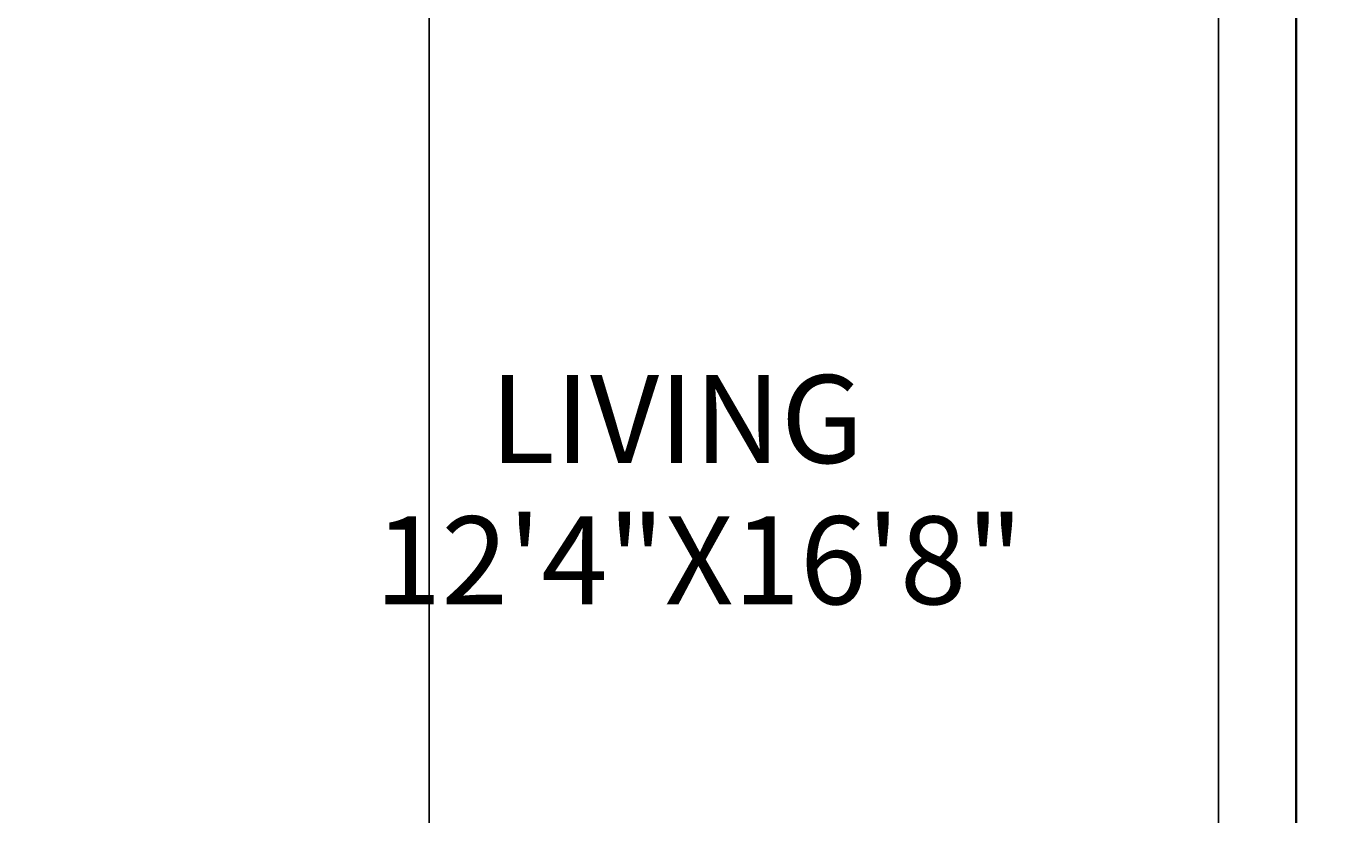
# Model space of a CAD drawing. Units: feet. Extents: x 5816 to 6644, y 25475 to 26788.
# Tile 9 of 23: x 6052 to 6232, y 26265 to 26373. Entities that reach past the tile are written whole.
import ezdxf

# ---------------------------------------------------------------- set-up
doc = ezdxf.new("R2010")
doc.units = ezdxf.units.FT
for name, color, linetype, lineweight in [('A-ANNO-DIMS', 2, 'Continuous', 13), ('A-AREA-IDEN', 7, 'Continuous', 18), ('A-WALL', 7, 'Continuous', 35)]:
    doc.layers.add(name, color=color, linetype=linetype, lineweight=lineweight)
doc.styles.get("Standard").update_dxf_attribs({"font": 'arial.ttf'})
doc.dimstyles.get("Standard").update_dxf_attribs({"dimtxt": 0.18, "dimasz": 0.18, "dimexe": 0.18, "dimexo": 0.0625, "dimgap": 0.09, "dimtad": 0, "dimtih": 1, "dimtoh": 1, "dimdec": 4, "dimzin": 0, "dimdsep": 46, "dimtxsty": 'Standard', "dimcen": 0.09, "dimadec": 0, "dimazin": 0, "dimtfac": 1, "dimtdec": 4, "dimtofl": 0, "dimtmove": 0, "dimatfit": 3, "dimfxl": 1, "dimtolj": 1, "dimtzin": 0, "dimarcsym": 0})

# ---------------------------------------------------------------- blocks, each defined once
blk = doc.blocks.new('*D58')
at = {"layer": 'A-ANNO-DIMS', "color": 0, "lineweight": -2, "transparency": 16777216}
for p, q in [((5953.98, 26168.65), (5953.98, 26787.91)), ((5954.16, 26787.73), (6030.2, 26787.73)), ((6106.8, 26787.73), (6030.76, 26787.73)), ((6106.98, 26168.71), (6106.98, 26787.91))]:
    blk.add_line(p, q, dxfattribs=at)
at = {"layer": 'A-ANNO-DIMS', "color": 0, "transparency": 16777216}
for points in [[(5954.16, 26787.76), (5954.16, 26787.7), (5953.98, 26787.73)], [(6106.8, 26787.76), (6106.8, 26787.7), (6106.98, 26787.73)]]:
    blk.add_solid(points, dxfattribs=at)
at = {"layer": 'Defpoints', "color": 0, "transparency": 16777216}
for p in [(6106.98, 26787.73), (5953.98, 26168.58), (6106.98, 26168.65)]:
    blk.add_point(p, dxfattribs=at)
at = {"layer": 'A-ANNO-DIMS', "color": 0, "transparency": 16777216, "insert": (6030.48, 26787.73), "char_height": 0.18, "attachment_point": 5}
blk.add_mtext('\\A1;153', dxfattribs=at)
blk = doc.blocks.new('*D60')
at = {"layer": 'A-ANNO-DIMS', "color": 0, "lineweight": -2, "transparency": 16777216}
for p, q in [((6106.98, 26094.4), (6106.98, 26787.91)), ((6107.16, 26787.73), (6224.93, 26787.73)), ((6343.5, 26787.73), (6225.72, 26787.73)), ((6343.68, 26094.4), (6343.68, 26787.91))]:
    blk.add_line(p, q, dxfattribs=at)
at = {"layer": 'A-ANNO-DIMS', "color": 0, "transparency": 16777216}
for points in [[(6107.16, 26787.76), (6107.16, 26787.7), (6106.98, 26787.73)], [(6343.5, 26787.76), (6343.5, 26787.7), (6343.68, 26787.73)]]:
    blk.add_solid(points, dxfattribs=at)
at = {"layer": 'Defpoints', "color": 0, "transparency": 16777216}
for p in [(6343.68, 26787.73), (6106.98, 26094.34), (6343.68, 26094.34)]:
    blk.add_point(p, dxfattribs=at)
at = {"layer": 'A-ANNO-DIMS', "color": 0, "transparency": 16777216, "insert": (6225.33, 26787.73), "char_height": 0.18, "attachment_point": 5}
blk.add_mtext('\\A1;236.7', dxfattribs=at)
blk = doc.blocks.new('*D72')
at = {"layer": 'A-ANNO-DIMS', "color": 0, "lineweight": -2, "transparency": 16777216}
for p, q in [((6214.69, 26168.65), (6214.69, 26787.91)), ((6214.87, 26787.73), (6219.56, 26787.73)), ((6225.13, 26787.73), (6220.44, 26787.73)), ((6225.31, 26177.65), (6225.31, 26787.91))]:
    blk.add_line(p, q, dxfattribs=at)
at = {"layer": 'A-ANNO-DIMS', "color": 0, "transparency": 16777216}
for points in [[(6214.87, 26787.76), (6214.87, 26787.7), (6214.69, 26787.73)], [(6225.13, 26787.76), (6225.13, 26787.7), (6225.31, 26787.73)]]:
    blk.add_solid(points, dxfattribs=at)
at = {"layer": 'Defpoints', "color": 0, "transparency": 16777216}
for p in [(6225.31, 26787.73), (6225.31, 26177.58), (6214.69, 26168.58)]:
    blk.add_point(p, dxfattribs=at)
at = {"layer": 'A-ANNO-DIMS', "color": 0, "transparency": 16777216, "insert": (6220, 26787.73), "char_height": 0.18, "attachment_point": 5}
blk.add_mtext('\\A1;10.621', dxfattribs=at)

msp = doc.modelspace()

# ---------------------------------------------------------------- linework, layer by layer
at = {"layer": 'A-WALL'}
msp.add_line((6225.3119, 26391.0846), (6225.3119, 26177.5846), dxfattribs=at)

# ---------------------------------------------------------------- texts
at = {"layer": 'A-ANNO-DIMS'}
msp.add_text('12\'4"X16\'8"', height=12, dxfattribs=at).set_placement((6099.5423, 26294.0714))
at = {"layer": 'A-AREA-IDEN'}
msp.add_text('LIVING', height=12, dxfattribs=at).set_placement((6115.2321, 26313.3484))

# ---------------------------------------------------------------- dimensions: what is measured, and where the dimension line sits
at = {"layer": 'A-ANNO-DIMS'}
for base, p1, p2, override, picture, middle in [((6106.9781, 26787.7346), (5953.9781, 26168.5846), (6106.9781, 26168.6509), {"dimdec": 0, "dimlfac": 1, "dimrnd": 0, "dimzin": 0, "dimdsep": 46, "dimlunit": 2}, '*D58', (6030.4781, 26787.7346)), ((6343.6763, 26787.7346), (6106.9781, 26094.3368), (6343.6763, 26094.3368), {"dimdec": 1, "dimlfac": 1, "dimrnd": 0, "dimzin": 0, "dimdsep": 46, "dimlunit": 2}, '*D60', (6225.3272, 26787.7346)), ((6225.3119, 26787.7346), (6214.6905, 26168.5846), (6225.3119, 26177.5846), {"dimdec": 3, "dimlfac": 1, "dimrnd": 0, "dimzin": 0, "dimdsep": 46, "dimlunit": 2}, '*D72', (6220.0012, 26787.7346))]:
    dim = msp.add_linear_dim(base=base, p1=p1, p2=p2, dimstyle='Standard', override=override, dxfattribs=at)
    dim.commit()
    dim.dimension.update_dxf_attribs({"geometry": picture, "text_midpoint": middle})

doc.saveas('drawing.dxf')
